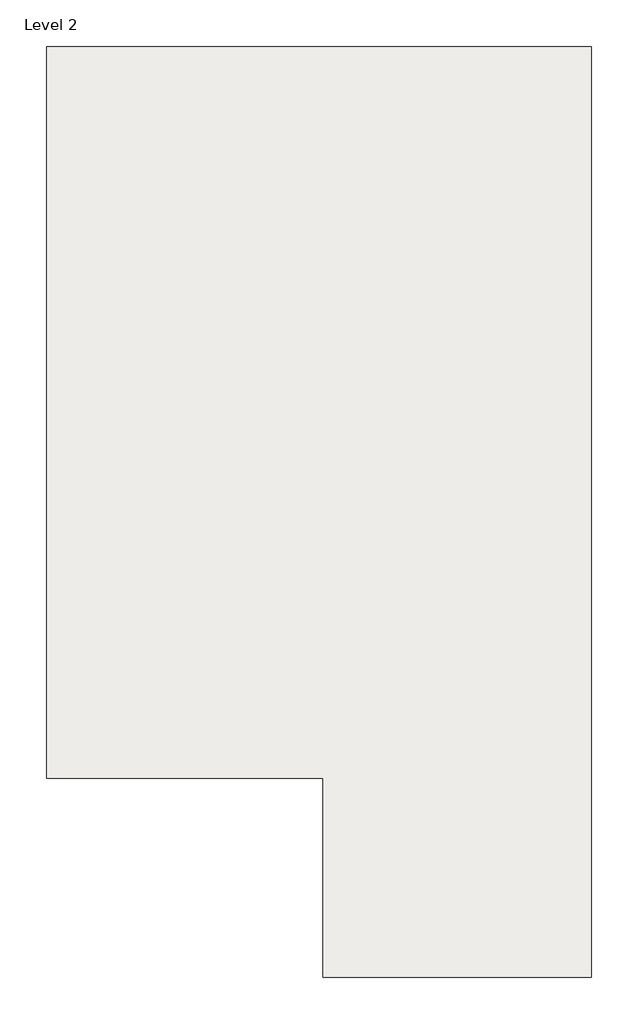
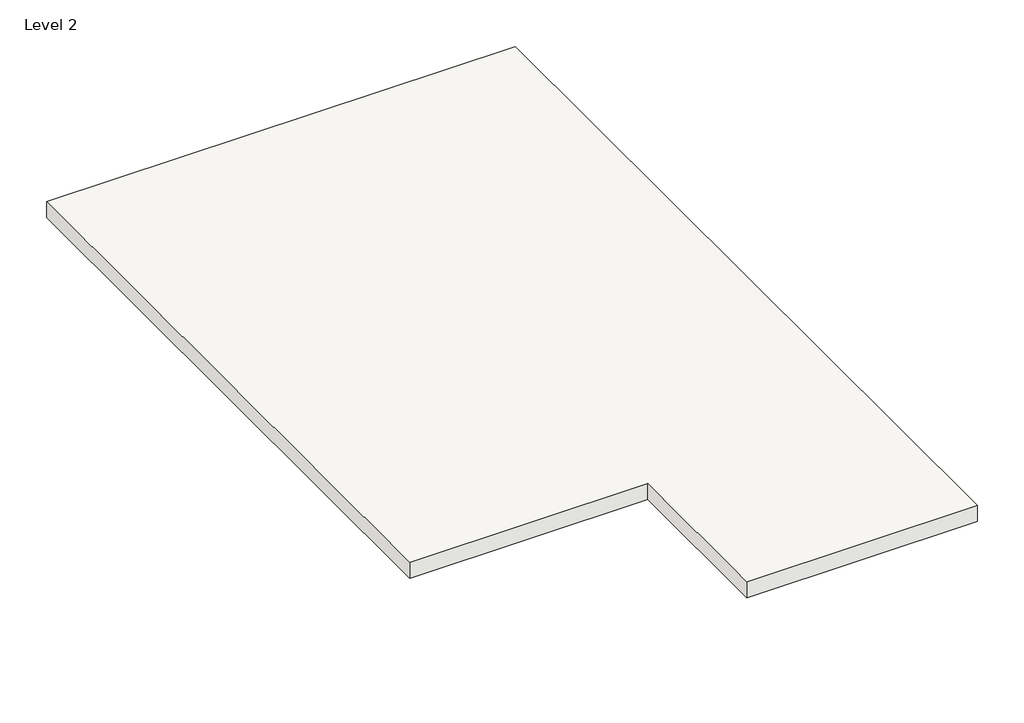
# One storey: 1 roof.
"""IFC4 building model written with IfcOpenShell, lengths in millimetres."""

from ifc_helpers import new_model, si_unit, frame, origin, place, context, project, spatial, polyline, outline, extrude, element, save

model = new_model("IFC4")

# Units and contexts
model_context = context("Model", 3, world=origin())
ifc_project = project(units=[si_unit("LENGTHUNIT", "METRE", prefix="MILLI")], contexts=[model_context])

# Site, building, storey
site = spatial("IfcSite", under=ifc_project)
building = spatial("IfcBuilding", under=site)
storey = spatial("IfcBuildingStorey", under=building, Name="Level 2", Elevation=3048.0)

# Roof
placement = place(None, origin())
element("IfcRoof", 1, ObjectType="Generic - 12\"", at=placement, inside=storey, context=model_context, shape_type="SweptSolid", body=[
    extrude(outline(polyline([(-16390.3267032, 13410.3187882), (-7982.9267032, 13410.3187882), (-7982.9267032, -940.6812118), (-12123.1267032, -940.6812118), (-12123.1267032, 2132.7187882), (-16390.3267032, 2132.7187882), (-16390.3267032, 13410.3187882)])), frame((0.0, 0.0, 3048.0), z_axis=(0.0, 0.0, 1.0), x_axis=(1.0, 0.0, 0.0)), (0.0, 0.0, 1.0), 304.8),
])

save(model, "model.ifc")

# Revit data of these elements
# Type "Generic - 12\""
#   Assembly Code = "B1020"
#   Layers, outside or top first: 1' - 0" "Brick, Soldier Course" (function 1)
# Element 1 (IfcRoof, "Generic - 12\"")
#   built-in parameter 1001705 = 11 (stored number, unit not read)
#   built-in parameter 1001710 = 33615
#   Phase Created = New Construction
#   Materials on its faces: "Brick, Soldier Course"
# Materials
#   "Brick, Soldier Course": class "Masonry", colour RGB 170 98 104, transparency 0, Description = "Common brick soldier coursed", Cost = 0
